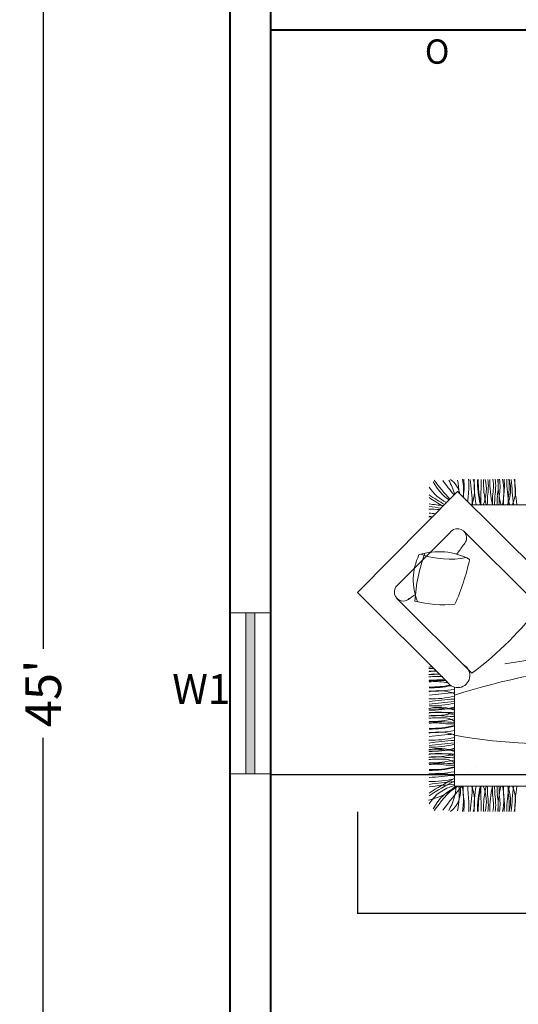
# Model space of a CAD drawing. Units: inches. Extents: x 182 to 1022, y -617 to 111.
# Tile 2 of 33: x 182 to 294, y -340 to -120. Entities that reach past the tile are written whole.
import ezdxf

# ---------------------------------------------------------------- set-up
doc = ezdxf.new("R2010")
doc.units = ezdxf.units.IN
doc.header["$MEASUREMENT"] = 0
for name, color, linetype, lineweight in [('A-ANNO-DIMS', 2, 'Continuous', 18), ('A-ANNO-IDEN', 1, 'Continuous', 18), ('A-GLAZ-PATT', 5, 'Continuous', 13), ('wall', 1, 'Continuous', 40), ('wind', 5, 'Continuous', 20)]:
    doc.layers.add(name, color=color, linetype=linetype, lineweight=lineweight)
doc.layers.add('furniture', color=50, linetype='Continuous', lineweight=15, transparency=0.8)
doc.styles.get("Standard").update_dxf_attribs({"font": 'arial.ttf'})
doc.dimstyles.get("Standard").update_dxf_attribs({"dimtxt": 0.18, "dimasz": 0.18, "dimexe": 0.18, "dimexo": 0.0625, "dimgap": 0.09, "dimtad": 0, "dimtih": 1, "dimtoh": 1, "dimdec": 1, "dimzin": 0, "dimdsep": 46, "dimlunit": 4, "dimtxsty": 'Standard', "dimcen": 0.09, "dimadec": 0, "dimazin": 0, "dimtfac": 1, "dimtdec": 1, "dimtofl": 0, "dimtmove": 0, "dimatfit": 3, "dimfxl": 1, "dimtolj": 1, "dimtzin": 0, "dimarcsym": 0})

# ---------------------------------------------------------------- blocks, each defined once
blk = doc.blocks.new('_ArchTick')
at = {"color": 0, "linetype": 'ByBlock', "const_width": 0.15}
blk.add_lwpolyline([(-0.5, -0.5), (0.5, 0.5)], dxfattribs=at)
blk = doc.blocks.new('*D6')
at = {"layer": 'A-ANNO-DIMS', "color": 0, "lineweight": -2, "transparency": 16777216}
for p, q in [((187.47, -0.37), (187.47, -260.42)), ((187.47, -540.37), (187.47, -280.32))]:
    blk.add_line(p, q, dxfattribs=at)
at = {"layer": 'Defpoints', "color": 0, "transparency": 16777216}
for p in [(229.36, -0.37), (187.47, -540.37), (229.36, -540.37)]:
    blk.add_point(p, dxfattribs=at)
at = {"layer": 'A-ANNO-DIMS', "color": 0, "lineweight": -2, "transparency": 16777216, "xscale": 8, "yscale": 8, "zscale": 8}
for p, rotation in [((187.47, -0.37), 90), ((187.47, -540.37), 270)]:
    blk.add_blockref('_ArchTick', p, dxfattribs=dict(at, rotation=rotation))
at = {"layer": 'A-ANNO-DIMS', "color": 0, "transparency": 16777216, "insert": (187.47, -270.37), "char_height": 8, "attachment_point": 5, "rotation": 90}
blk.add_mtext("\\A1;45'", dxfattribs=at)
blk = doc.blocks.new('LOUNGE-SEATING-GROUP')
for p, q in [((22.37, 71.64), (0, 48.98)), ((22.37, 71.64), (42.71, 51.42)), ((23.45, 70.43), (23.45, 70.43)), ((23.45, 70.43), (23.45, 70.43)), ((23.45, 70.43), (23.45, 70.43)), ((24.81, 70.1), (24.81, 70.1)), ((24.81, 70.1), (24.81, 70.1)), ((24.81, 70.1), (24.81, 70.1)), ((25.37, 68.66), (46.02, 68.66)), ((27.79, 69.24), (27.79, 69.24)), ((27.79, 69.24), (27.79, 69.24)), ((32.6, 69.72), (32.6, 69.72)), ((34.6, 69.02), (34.6, 69.02)), ((29.83, 67.31), (29.83, 67.31)), ((29.68, 65.32), (29.68, 65.32)), ((20.57, 62.3), (8.95, 50.67)), ((20.57, 62.3), (16.28, 58)), ((23.81, 62.71), (38.96, 47.66)), ((12.73, 54.45), (8.95, 50.67)), ((0, 48.98), (20.08, 29.02)), ((25.6, 30.99), (8.82, 47.69)), ((21.66, 5.69), (21.66, 27.82)), ((18.1, 23.39), (18.1, 23.39)), ((18.64, 23.43), (18.64, 23.43)), ((18.1, 14.15), (18.1, 14.15)), ((18.64, 14.19), (18.64, 14.19)), ((26.54, 9.97), (26.54, 9.97)), ((24.84, 8.76), (24.84, 8.76)), ((134.14, 5.69), (21.66, 5.69)), ((23.45, 3.92), (23.45, 3.92)), ((23.45, 3.92), (23.45, 3.92)), ((23.45, 3.92), (23.45, 3.92)), ((24.81, 4.25), (24.81, 4.25)), ((24.81, 4.25), (24.81, 4.25)), ((24.81, 4.25), (24.81, 4.25))]:
    blk.add_line(p, q)
for centre, radius, start, end in [((26.62, 78.75), 10.9, 207.3033, 235.7016), ((48.18, 96.13), 38.02, 215.3153, 223.6457), ((157.47, 180.45), 174.58, 217.5441, 218.8901), ((9.21, 67.69), 12.92, 14.6792, 29.865), ((17.54, 69.88), 5.5, 12.9777, 54.0943), ((7.21, 70.59), 15.55, 2.5322, 13.2785), ((9.4, 71.55), 14.33, 355.1756, 11.2455), ((11.06, 72.81), 12.79, 349.9349, 6.8829), ((12.13, 72.82), 12.79, 349.9349, 6.8829), ((-225.09, 48.88), 251.6, 4.5146, 5.8017), ((17.36, 72.06), 8.84, 337.3098, 14.8613), ((54.69, 73.85), 28.62, 179.0195, 190.4039), ((48.4, 73.82), 21.55, 178.6331, 193.8573), ((48.56, 73.82), 21.55, 178.6331, 193.8573), ((-156.89, 73.02), 184.52, 358.628, 0.3934), ((19.99, 72.06), 8.84, 337.3098, 14.8613), ((49.71, 73.82), 21.55, 178.6331, 193.8573), ((16.48, 72.8), 12.79, 349.9349, 6.8829), ((51.14, 73.82), 21.55, 178.6331, 193.8573), ((17.61, 72.81), 12.79, 349.9349, 6.8829), ((18.12, 72.81), 12.79, 349.9349, 6.8829), ((18.68, 72.81), 12.79, 349.9349, 6.8829), ((52.99, 73.83), 21.55, 178.6331, 193.8573), ((19.1, 72.81), 12.79, 349.9349, 6.8829), ((18.41, 71.55), 14.33, 348.4112, 11.2455), ((20.08, 72.81), 12.79, 349.9349, 6.8829), ((54.95, 73.83), 21.55, 178.6331, 193.8573), ((25.41, 72.08), 8.84, 337.3098, 14.8613), ((21.15, 72.82), 12.79, 349.9349, 6.8829), ((-215.95, 48.88), 251.6, 4.5146, 5.8017), ((26.5, 72.06), 8.84, 337.3098, 14.8613), ((63.83, 73.85), 28.62, 179.0195, 190.4039), ((50.72, 123.93), 63.44, 236.8219, 240.5026), ((23.91, 77.56), 9.3, 212.2712, 244.6274), ((167.37, 66.07), 142.71, 178.1891, 178.6709), ((171.72, 66.06), 142.71, 178.1891, 178.9775), ((172.85, 66.06), 142.71, 178.1891, 178.9775), ((173.36, 66.06), 142.71, 178.1891, 178.9775), ((173.92, 66.06), 142.71, 178.1891, 178.9775), ((174.34, 66.06), 142.71, 178.1891, 178.9775), ((175.32, 66.07), 142.71, 178.1891, 178.9775), ((176.39, 66.07), 142.71, 178.1891, 178.9775), ((50.71, 123.35), 63.44, 236.8219, 240.1356), ((25.24, 129.76), 61.61, 261.3771, 264.3888), ((16.49, 46.09), 21.55, 85.0538, 91.3669), ((25.23, 129.18), 61.61, 261.3771, 263.9203), ((41.44, 317.08), 251.6, 264.1983, 264.5236), ((16.47, 37.31), 28.62, 89.4753, 90.9805), ((18.26, 74.63), 8.84, 255.1387, 260.0752), ((22.35, 61.25), 2.06, 307.6748, 149.5181), ((-9.78, 81.21), 39.77, 323.5454, 327.1144), ((25.49, 51.8), 13.03, 154.4501, 201.7699), ((47.31, 45.46), 34.51, 159.0815, 177.2768), ((18.23, 43.53), 14.61, 62.0126, 107.9429), ((20.65, 76.24), 19.77, 250.9005, 280.6513), ((-28.28, 68.33), 54.68, 336.3371, 347.4176), ((10.26, 49.12), 2.03, 130.1092, 319.8908), ((-9.78, 81.21), 39.77, 301.0867, 304.727), ((19.32, 71.82), 25.56, 255.3068, 275.5663), ((-19.25, 91.37), 75.22, 306.6049, 323.3387), ((76.48, -220.38), 257.15, 94.6196, 99.7513), ((16.49, 53.56), 21.55, 268.6331, 271.5238), ((18.24, 22.68), 8.84, 94.2757, 104.8613), ((16.51, 54.45), 21.55, 268.6331, 269.1046), ((18.25, 23.77), 8.84, 100.6592, 104.8613), ((17.52, 19.64), 12.79, 93.8173, 96.8829), ((17.3, -153.11), 184.52, 89.8849, 90.3934), ((22.4, 30.44), 2.72, 211.4693, 56.9076), ((71.51, -132.24), 165.96, 95.4421, 107.4799), ((16.49, 52.22), 21.55, 268.6331, 274.9238), ((17.51, 17.97), 12.79, 86.2453, 96.8829), ((18.22, 10.3), 19.94, 87.4435, 96.4413), ((16.5, 50.95), 21.55, 268.6331, 277.9798), ((18.27, 0.21), 29.12, 86.9677, 94.5064), ((17.52, 16.29), 12.79, 79.9349, 96.8829), ((24.26, 171.53), 142.71, 268.1891, 268.3576), ((16.47, 55.53), 28.62, 269.0195, 280.4039), ((16.5, 49.41), 21.55, 268.6331, 281.3519), ((16.5, 49.25), 21.55, 268.6331, 281.8302), ((18.26, 18.21), 8.84, 67.3098, 104.8613), ((41.44, -224.24), 251.6, 94.5146, 95.8017), ((16.49, 46.75), 21.55, 268.6331, 283.8573), ((25.23, -36.35), 61.61, 93.3644, 98.6229), ((16.51, 45.2), 21.55, 268.6331, 283.8573), ((25.24, -36.92), 61.61, 93.3644, 98.6229), ((16.49, 44.31), 21.55, 268.6331, 283.8573), ((18.24, 13.43), 8.84, 67.3098, 104.8613), ((16.49, 42.97), 21.55, 268.6331, 283.8573), ((18.25, 14.52), 8.84, 67.3098, 104.8613), ((16.5, 44.24), 21.55, 268.6331, 283.8573), ((17.52, 10.39), 12.79, 79.9349, 96.8829), ((17.3, -162.36), 184.52, 88.628, 90.3934), ((24.27, 165.63), 142.71, 268.1891, 268.9775), ((17.51, 8.72), 12.79, 79.9349, 96.8829), ((18.22, 1.05), 19.94, 87.4435, 96.4413), ((16.5, 41.7), 21.55, 268.6331, 283.8573), ((18.27, -9.04), 29.12, 83.3702, 94.5064), ((17.52, 7.04), 12.79, 79.9349, 96.8829), ((19.32, 17.13), 3.85, 51.6564, 93.1744), ((24.26, 163.96), 142.71, 268.1891, 268.9775), ((16.47, 46.28), 28.62, 269.0195, 280.4039), ((16.5, 40.16), 21.55, 268.6331, 283.8573), ((16.5, 40), 21.55, 268.6331, 283.8573), ((18.26, 8.96), 8.84, 67.3098, 104.8613), ((24.26, 162.28), 142.71, 268.1891, 268.9775), ((16.49, 37.5), 21.55, 268.6331, 283.8573), ((25.23, -45.6), 61.61, 93.3644, 98.6229), ((41.44, -233.49), 251.6, 94.5146, 95.8017), ((43.3, 138.88), 123.73, 259.9275, 281.2246), ((16.49, 35.07), 21.55, 268.6331, 283.8573), ((16.51, 35.96), 21.55, 268.6331, 283.8573), ((18.25, 5.28), 8.84, 67.3098, 104.8613), ((16.5, 35), 21.55, 268.6331, 283.8573), ((17.52, 1.15), 12.79, 79.9349, 96.8829), ((25.24, -46.17), 61.61, 93.3644, 98.6229), ((24.27, 156.39), 142.71, 268.1891, 268.9775), ((18.24, 4.2), 8.84, 67.3098, 104.8613), ((16.49, 33.73), 21.55, 268.6331, 283.8573), ((17.51, -0.52), 12.79, 79.9349, 96.8829), ((18.22, -8.19), 19.94, 87.4435, 96.4413), ((16.5, 32.46), 21.55, 268.6331, 283.8573), ((17.3, -171.6), 184.52, 88.628, 90.3934), ((19.32, 7.89), 3.85, 51.6564, 93.1744), ((24.26, 154.72), 142.71, 268.1891, 268.9775), ((18.27, -18.28), 29.12, 83.3702, 94.5064), ((17.52, -2.2), 12.79, 79.9349, 96.8829), ((16.47, 37.04), 28.62, 269.0195, 280.4039), ((16.5, 30.92), 21.55, 268.6331, 283.8573), ((16.5, 30.76), 21.55, 268.6331, 283.8573), ((24.26, 153.04), 142.71, 268.1891, 268.9775), ((16.49, 28.26), 21.55, 268.6331, 283.8573), ((18.26, -0.28), 8.84, 67.3098, 104.8613), ((50.71, -49), 63.44, 117.2669, 123.1781), ((25.23, -54.84), 61.61, 93.3644, 98.6229), ((41.44, -242.73), 251.6, 94.5146, 95.8017), ((50.72, -49.58), 63.44, 117.2669, 123.1781), ((12.09, 18.89), 16.76, 282.9523, 308.0769), ((25.24, -55.41), 61.61, 93.3644, 98.6229), ((23.91, -3.21), 9.3, 103.9935, 147.7288), ((26.62, -4.4), 10.9, 112.1181, 152.6967), ((48.18, -21.78), 38.02, 133.716, 144.6847), ((157.47, -106.1), 174.58, 140.1568, 142.4559), ((9.21, 6.66), 12.92, 330.135, 355.7243), ((17.54, 4.47), 5.5, 305.9057, 12.8054), ((7.21, 3.76), 15.55, 346.7215, 7.1491), ((9.4, 2.8), 14.33, 348.7545, 11.5888), ((166.3, 8.28), 142.71, 181.0225, 181.8109), ((167.37, 8.28), 142.71, 181.0225, 181.8109), ((-225.09, 25.47), 251.6, 354.1983, 355.4854), ((17.36, 2.29), 8.84, 345.1387, 22.6902), ((54.69, 0.5), 28.62, 169.5961, 180.9805), ((48.4, 0.53), 21.55, 166.1427, 181.3669), ((48.56, 0.53), 21.55, 166.1427, 181.3669), ((-156.89, 1.33), 184.52, 359.6066, 1.372), ((19.99, 2.28), 8.84, 345.1387, 22.6902), ((49.71, 0.53), 21.55, 166.1427, 181.3669), ((171.72, 8.29), 142.71, 181.0225, 181.8109), ((51.14, 0.53), 21.55, 166.1427, 181.3669), ((172.85, 8.29), 142.71, 181.0225, 181.8109), ((173.36, 8.29), 142.71, 181.0225, 181.8109), ((173.92, 8.29), 142.71, 181.0225, 181.8109), ((52.99, 0.52), 21.55, 166.1427, 181.3669), ((174.34, 8.28), 142.71, 181.0225, 181.8109), ((18.41, 2.8), 14.33, 348.7545, 11.5888), ((175.32, 8.28), 142.71, 181.0225, 181.8109), ((54.95, 0.52), 21.55, 166.1427, 181.3669), ((25.41, 2.27), 8.84, 345.1387, 22.6902), ((176.39, 8.28), 142.71, 181.0225, 181.8109), ((-215.95, 25.47), 251.6, 354.1983, 355.4854), ((26.5, 2.29), 8.84, 345.1387, 22.6902), ((63.83, 0.5), 28.62, 169.5961, 180.9805), ((11.06, 1.54), 12.79, 353.1171, 10.0651), ((12.13, 1.53), 12.79, 353.1171, 10.0651), ((16.48, 1.55), 12.79, 353.1171, 10.0651), ((17.61, 1.54), 12.79, 353.1171, 10.0651), ((18.12, 1.54), 12.79, 353.1171, 10.0651), ((18.68, 1.54), 12.79, 353.1171, 10.0651), ((19.1, 1.54), 12.79, 353.1171, 10.0651), ((20.08, 1.54), 12.79, 353.1171, 10.0651), ((21.15, 1.53), 12.79, 353.1171, 10.0651)]:
    blk.add_arc(centre, radius, start, end)
blk = doc.blocks.new('*D26')
at = {"layer": 'A-ANNO-DIMS', "color": 0, "lineweight": -2, "transparency": 16777216}
for p, q in [((257.85, -296.88), (257.85, -319.73)), ((409.39, -296.88), (409.39, -319.73)), ((258.03, -319.55), (331.64, -319.55)), ((409.21, -319.55), (335.59, -319.55))]:
    blk.add_line(p, q, dxfattribs=at)
at = {"layer": 'A-ANNO-DIMS', "color": 0, "transparency": 16777216}
for points in [[(258.03, -319.52), (258.03, -319.58), (257.85, -319.55)], [(409.21, -319.52), (409.21, -319.58), (409.39, -319.55)]]:
    blk.add_solid(points, dxfattribs=at)
at = {"layer": 'Defpoints', "color": 0, "transparency": 16777216}
for p in [(257.85, -296.82), (409.39, -296.82), (409.39, -319.55)]:
    blk.add_point(p, dxfattribs=at)
at = {"layer": 'A-ANNO-DIMS', "color": 0, "transparency": 16777216, "insert": (333.62, -319.55), "char_height": 0.18, "attachment_point": 5}
blk.add_mtext('\\A1;LOUNGE GROUP 12\'-7 1/2" TYP.', dxfattribs=at)
blk = doc.blocks.new('*D39')
at = {"layer": 'A-ANNO-DIMS', "color": 0, "lineweight": -2, "transparency": 16777216}
for p, q in [((238.4, -288.54), (1015.28, -288.54)), ((1015.1, -288.72), (1015.1, -346.77)), ((1015.1, -405.19), (1015.1, -347.14)), ((238.43, -405.37), (1015.28, -405.37))]:
    blk.add_line(p, q, dxfattribs=at)
at = {"layer": 'A-ANNO-DIMS', "color": 0, "transparency": 16777216}
for points in [[(1015.07, -288.72), (1015.13, -288.72), (1015.1, -288.54)], [(1015.07, -405.19), (1015.13, -405.19), (1015.1, -405.37)]]:
    blk.add_solid(points, dxfattribs=at)
at = {"layer": 'Defpoints', "color": 0, "transparency": 16777216}
for p in [(238.34, -288.54), (1015.1, -288.54), (238.36, -405.37)]:
    blk.add_point(p, dxfattribs=at)
at = {"layer": 'A-ANNO-DIMS', "color": 0, "transparency": 16777216, "insert": (1015.1, -346.96), "char_height": 0.18, "attachment_point": 5}
blk.add_mtext('\\A1;9\'-9"', dxfattribs=at)

msp = doc.modelspace()

# ---------------------------------------------------------------- hatches: boundary and pattern name
at = {"layer": 'A-GLAZ-PATT'}
h = msp.add_hatch(color=256, dxfattribs=at)
h.dxf.hatch_style = 1
h.paths.add_polyline_path([(285.4, -3.87), (255.4, -3.87), (255.4, -5.87), (285.4, -5.87)])
h.paths.add_polyline_path([(376.09, -3.87), (340.09, -3.87), (340.09, -5.87), (376.09, -5.87)])
h.paths.add_polyline_path([(561.86, -132.92), (559.86, -132.92), (559.86, -168.92), (561.86, -168.92)])
h.paths.add_polyline_path([(561.86, -56.81), (559.86, -56.81), (559.86, -86.81), (561.86, -86.81)])
h.paths.add_polyline_path([(561.86, -258.37), (559.86, -258.37), (559.86, -282.37), (561.86, -282.37)])
h.paths.add_polyline_path([(533.36, -534.87), (497.36, -534.87), (497.36, -536.87), (533.36, -536.87)])
h.paths.add_polyline_path([(234.86, -252.37), (232.86, -252.37), (232.86, -288.37), (234.86, -288.37)])

# ---------------------------------------------------------------- linework, layer by layer
at = {"layer": 'wall'}
for p, q in [((229.36, -540.37), (229.36, -0.37)), ((238.36, -9.37), (238.36, -540.37)), ((238.36, -121.87), (428.86, -121.87))]:
    msp.add_line(p, q, dxfattribs=at)
at = {"layer": 'wind'}
for p, q in [((229.36, -252.37), (238.36, -252.37)), ((232.86, -252.37), (232.86, -288.37)), ((234.86, -252.37), (234.86, -288.37)), ((229.36, -288.37), (238.36, -288.37))]:
    msp.add_line(p, q, dxfattribs=at)

# ---------------------------------------------------------------- block references
at = {"layer": 'furniture'}
msp.add_blockref('LOUNGE-SEATING-GROUP', (257.85, -296.82), dxfattribs=at)

# ---------------------------------------------------------------- texts
at = {"layer": 'A-ANNO-IDEN'}
for s, height, p in [('O', 5.44, (272.91, -129.48)), ('W1', 6.652, (216.37, -272.73))]:
    msp.add_text(s, height=height, dxfattribs=at).set_placement(p)

# ---------------------------------------------------------------- dimensions: what is measured, and where the dimension line sits
at = {"layer": 'A-ANNO-DIMS'}
for base, p1, p2, override, picture, middle in [((187.47, -540.37), (229.36, -0.37), (229.36, -540.37), {"dimtxt": 8, "dimasz": 8, "dimgap": 3, "dimtih": 0, "dimblk1": 'ArchTick', "dimblk2": 'ArchTick', "dimsah": 1, "dimse1": 1, "dimse2": 1, "dimclrd": 0, "dimclre": 0, "dimclrt": 0}, '*D6', (187.47, -270.37)), ((1015.1, -288.54), (238.36, -405.37), (238.34, -288.54), {"dimdec": 1, "dimlfac": 1, "dimrnd": 0, "dimzin": 1, "dimdsep": 46, "dimlunit": 4, "dimfrac": 2}, '*D39', (1015.1, -346.96))]:
    dim = msp.add_linear_dim(base=base, p1=p1, p2=p2, angle=90, dimstyle='Standard', override=override, dxfattribs=at)
    dim.commit()
    dim.dimension.update_dxf_attribs({"geometry": picture, "text_midpoint": middle})
dim = msp.add_linear_dim(base=(409.39, -319.55), p1=(257.85, -296.82), p2=(409.39, -296.82), text='LOUNGE GROUP <> TYP.', dimstyle='Standard', override={"dimdec": 1, "dimlfac": 1, "dimrnd": 0, "dimzin": 1, "dimdsep": 46, "dimlunit": 4, "dimfrac": 2}, dxfattribs=at)
dim.commit()
dim.dimension.update_dxf_attribs({"geometry": '*D26', "text_midpoint": (333.62, -319.55)})

doc.saveas('drawing.dxf')
